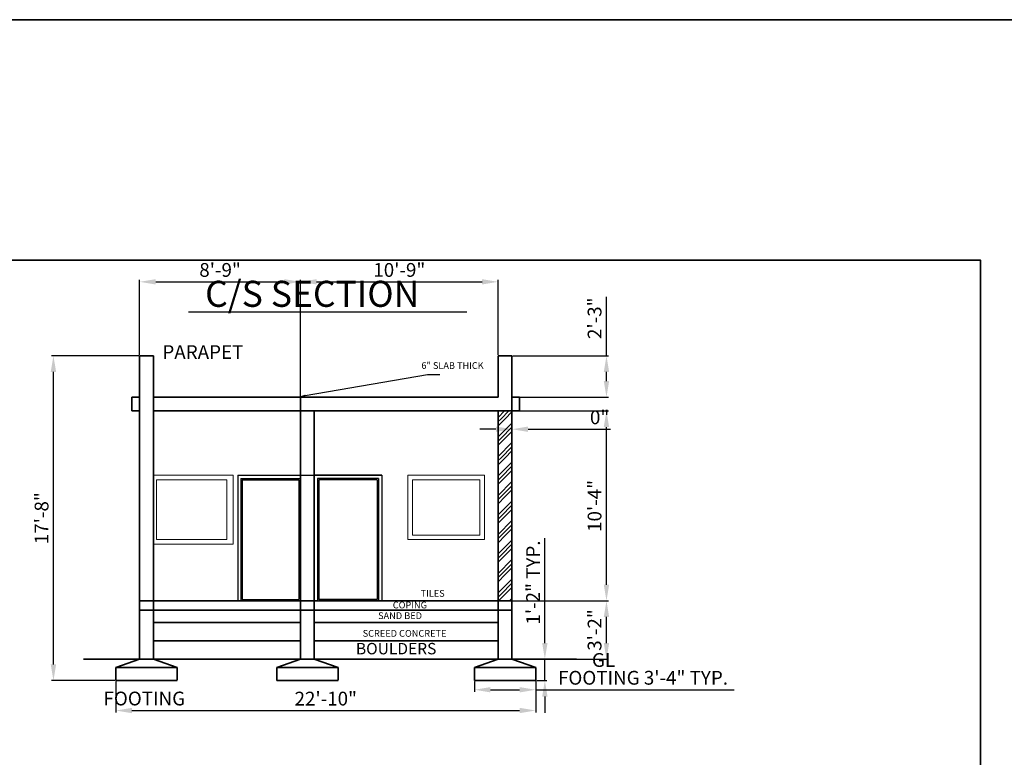
# Model space of a CAD drawing. Units: inches. Extents: x 1956 to 4770, y 1551 to 2596.
# Tile 9 of 10: x 2667 to 3310, y 2115 to 2596. Entities that reach past the tile are written whole.
import ezdxf
from ezdxf import colors
from ezdxf.entities.mleader import LeaderData, LeaderLine
from ezdxf.math import Vec2, Vec3

# ---------------------------------------------------------------- set-up
doc = ezdxf.new("R2010")
doc.units = ezdxf.units.IN
for name, color, linetype, lineweight in [('A-ANNO-DIMS', 2, 'Continuous', 18), ('A-ANNO-TEXT', 7, 'Continuous', 18), ('A-ANNO-TITL', 6, 'Continuous', 25), ('A-ANNO-TTLB', 7, 'Continuous', 35), ('A-DOOR', 3, 'Continuous', 25), ('A-GLAZ', 4, 'Continuous', 18), ('A-SECT', 7, 'Continuous', 35), ('A-SECT-PATT', 8, 'Continuous', 13), ('S-FNDN', 7, 'Continuous', 35)]:
    doc.layers.add(name, color=color, linetype=linetype, lineweight=lineweight)
doc.styles.get("Standard").update_dxf_attribs({"font": 'arial.ttf'})
doc.dimstyles.new('ISO-25', dxfattribs={"dimtxt": 9, "dimasz": 10.5, "dimexe": 1.25, "dimexo": 0.625, "dimgap": 2, "dimtad": 1, "dimdec": 1, "dimlunit": 4, "dimtxsty": 'Standard', "dimcen": 2.5, "dimadec": 0, "dimazin": 0, "dimtfac": 1, "dimtdec": 1, "dimtmove": 0, "dimatfit": 3, "dimfxl": 1, "dimarcsym": 0})

# ---------------------------------------------------------------- blocks, each defined once
blk = doc.blocks.new('*D15')
at = {"layer": 'A-ANNO-DIMS', "color": 0, "lineweight": -2, "transparency": 16777216}
for p, q in [((2988.15, 2340.24), (2988.15, 2327.69)), ((2988.15, 2340.24), (2988.15, 2327.69)), ((2977.65, 2328.94), (2967.15, 2328.94)), ((2998.65, 2328.94), (3052.57, 2328.94))]:
    blk.add_line(p, q, dxfattribs=at)
at = {"layer": 'A-ANNO-DIMS', "color": 0, "transparency": 16777216}
for points in [[(2977.65, 2330.69), (2977.65, 2327.19), (2988.15, 2328.94)], [(2998.65, 2330.69), (2998.65, 2327.19), (2988.15, 2328.94)]]:
    blk.add_solid(points, dxfattribs=at)
at = {"layer": 'Defpoints', "color": 0, "transparency": 16777216}
for p in [(2988.15, 2340.86), (2988.15, 2340.86), (2988.15, 2328.94)]:
    blk.add_point(p, dxfattribs=at)
at = {"layer": 'A-ANNO-DIMS', "color": 0, "transparency": 16777216, "insert": (3045.4, 2335.53), "char_height": 9, "attachment_point": 5}
blk.add_mtext('0"', dxfattribs=at)
blk = doc.blocks.new('FOOTING-40IN-SECTION')
for p, q in [((15.5, 14), (0, 8.58)), ((15.5, 14), (24.5, 14)), ((15.5, 14), (24.5, 14)), ((24.5, 14), (40, 8.58)), ((0, 8.58), (0, 7.18)), ((0, 8.58), (40, 8.58)), ((0, 7.18), (0, 0)), ((40, 8.58), (40, 7.18)), ((40, 7.18), (40, 0.18)), ((0, 0), (40, 0)), ((0, 0), (7.37, 0))]:
    blk.add_line(p, q)
blk = doc.blocks.new('*D37')
at = {"layer": 'A-ANNO-DIMS', "color": 0, "lineweight": -2, "transparency": 16777216}
for p, q in [((2963.65, 2164.24), (2963.65, 2157.61)), ((3003.65, 2164.24), (3003.65, 2157.61)), ((2974.15, 2158.86), (2993.15, 2158.86)), ((3003.65, 2158.86), (3133.27, 2158.86))]:
    blk.add_line(p, q, dxfattribs=at)
at = {"layer": 'A-ANNO-DIMS', "color": 0, "transparency": 16777216}
for points in [[(2974.15, 2160.61), (2974.15, 2157.11), (2963.65, 2158.86)], [(2993.15, 2160.61), (2993.15, 2157.11), (3003.65, 2158.86)]]:
    blk.add_solid(points, dxfattribs=at)
at = {"layer": 'Defpoints', "color": 0, "transparency": 16777216}
for p in [(2963.65, 2164.86), (3003.65, 2164.86), (3003.65, 2158.86)]:
    blk.add_point(p, dxfattribs=at)
at = {"layer": 'A-ANNO-DIMS', "color": 0, "transparency": 16777216, "insert": (3073.71, 2165.52), "char_height": 9, "attachment_point": 5}
blk.add_mtext('FOOTING 3\'-4" TYP.', dxfattribs=at)
blk = doc.blocks.new('*D38')
at = {"layer": 'A-ANNO-DIMS', "color": 0, "lineweight": -2, "transparency": 16777216}
for p, q in [((3009.65, 2189.36), (3009.65, 2257.88)), ((3004.28, 2178.86), (3010.9, 2178.86)), ((3009.65, 2164.86), (3009.65, 2178.86)), ((3004.28, 2164.86), (3010.9, 2164.86)), ((3009.65, 2154.36), (3009.65, 2143.86))]:
    blk.add_line(p, q, dxfattribs=at)
at = {"layer": 'A-ANNO-DIMS', "color": 0, "transparency": 16777216}
for points in [[(3007.9, 2189.36), (3011.4, 2189.36), (3009.65, 2178.86)], [(3007.9, 2154.36), (3011.4, 2154.36), (3009.65, 2164.86)]]:
    blk.add_solid(points, dxfattribs=at)
at = {"layer": 'Defpoints', "color": 0, "transparency": 16777216}
for p in [(3003.65, 2178.86), (3009.65, 2178.86), (3003.65, 2164.86)]:
    blk.add_point(p, dxfattribs=at)
at = {"layer": 'A-ANNO-DIMS', "color": 0, "transparency": 16777216, "insert": (3003.13, 2228.87), "char_height": 9, "attachment_point": 5, "rotation": 90}
blk.add_mtext('1\'-2" TYP.', dxfattribs=at)
blk = doc.blocks.new('*D80')
at = {"layer": 'A-ANNO-DIMS', "color": 0, "lineweight": -2, "transparency": 16777216}
for p, q in [((2729.65, 2164.24), (2729.65, 2144.06)), ((3003.65, 2164.24), (3003.65, 2144.06)), ((2740.15, 2145.31), (2993.15, 2145.31))]:
    blk.add_line(p, q, dxfattribs=at)
at = {"layer": 'A-ANNO-DIMS', "color": 0, "transparency": 16777216}
for points in [[(2740.15, 2147.06), (2740.15, 2143.56), (2729.65, 2145.31)], [(2993.15, 2147.06), (2993.15, 2143.56), (3003.65, 2145.31)]]:
    blk.add_solid(points, dxfattribs=at)
at = {"layer": 'Defpoints', "color": 0, "transparency": 16777216}
for p in [(2729.65, 2164.86), (3003.65, 2164.86), (3003.65, 2145.31)]:
    blk.add_point(p, dxfattribs=at)
at = {"layer": 'A-ANNO-DIMS', "color": 0, "transparency": 16777216, "insert": (2866.65, 2151.91), "char_height": 9, "attachment_point": 5}
blk.add_mtext('22\'-10"', dxfattribs=at)
blk = doc.blocks.new('*D81')
at = {"layer": 'A-ANNO-DIMS', "color": 0, "lineweight": -2, "transparency": 16777216}
for p, q in [((2744.53, 2376.86), (2687.64, 2376.86)), ((2688.89, 2175.36), (2688.89, 2366.36)), ((2729.03, 2164.86), (2687.64, 2164.86))]:
    blk.add_line(p, q, dxfattribs=at)
at = {"layer": 'A-ANNO-DIMS', "color": 0, "transparency": 16777216}
for points in [[(2687.14, 2366.36), (2690.64, 2366.36), (2688.89, 2376.86)], [(2687.14, 2175.36), (2690.64, 2175.36), (2688.89, 2164.86)]]:
    blk.add_solid(points, dxfattribs=at)
at = {"layer": 'Defpoints', "color": 0, "transparency": 16777216}
for p in [(2688.89, 2376.86), (2745.15, 2376.86), (2729.65, 2164.86)]:
    blk.add_point(p, dxfattribs=at)
at = {"layer": 'A-ANNO-DIMS', "color": 0, "transparency": 16777216, "insert": (2682.3, 2270.86), "char_height": 9, "attachment_point": 5, "rotation": 90}
blk.add_mtext('17\'-8"', dxfattribs=at)
blk = doc.blocks.new('*D82')
at = {"layer": 'A-ANNO-DIMS', "color": 0, "lineweight": -2, "transparency": 16777216}
for p, q in [((2988.78, 2340.86), (3051.11, 2340.86)), ((3049.86, 2227.36), (3049.86, 2330.36)), ((2988.78, 2216.86), (3051.11, 2216.86))]:
    blk.add_line(p, q, dxfattribs=at)
at = {"layer": 'A-ANNO-DIMS', "color": 0, "transparency": 16777216}
for points in [[(3048.11, 2330.36), (3051.61, 2330.36), (3049.86, 2340.86)], [(3048.11, 2227.36), (3051.61, 2227.36), (3049.86, 2216.86)]]:
    blk.add_solid(points, dxfattribs=at)
at = {"layer": 'Defpoints', "color": 0, "transparency": 16777216}
for p in [(2988.15, 2340.86), (3049.86, 2340.86), (2988.15, 2216.86)]:
    blk.add_point(p, dxfattribs=at)
at = {"layer": 'A-ANNO-DIMS', "color": 0, "transparency": 16777216, "insert": (3043.27, 2278.86), "char_height": 9, "attachment_point": 5, "rotation": 90}
blk.add_mtext('10\'-4"', dxfattribs=at)
blk = doc.blocks.new('*D83')
at = {"layer": 'A-ANNO-DIMS', "color": 0, "lineweight": -2, "transparency": 16777216}
for p, q in [((3049.86, 2376.86), (3049.86, 2415.44)), ((2988.78, 2376.86), (3051.11, 2376.86)), ((3049.86, 2360.36), (3049.86, 2366.36)), ((2988.78, 2349.86), (3051.11, 2349.86))]:
    blk.add_line(p, q, dxfattribs=at)
at = {"layer": 'A-ANNO-DIMS', "color": 0, "transparency": 16777216}
for points in [[(3048.11, 2366.36), (3051.61, 2366.36), (3049.86, 2376.86)], [(3048.11, 2360.36), (3051.61, 2360.36), (3049.86, 2349.86)]]:
    blk.add_solid(points, dxfattribs=at)
at = {"layer": 'Defpoints', "color": 0, "transparency": 16777216}
for p in [(2988.15, 2376.86), (3049.86, 2376.86), (2988.15, 2349.86)]:
    blk.add_point(p, dxfattribs=at)
at = {"layer": 'A-ANNO-DIMS', "color": 0, "transparency": 16777216, "insert": (3043.26, 2401.4), "char_height": 9, "attachment_point": 5, "rotation": 90}
blk.add_mtext('2\'-3"', dxfattribs=at)
blk = doc.blocks.new('*D84')
at = {"layer": 'A-ANNO-DIMS', "color": 0, "lineweight": -2, "transparency": 16777216}
for p, q in [((2988.78, 2216.86), (3051.11, 2216.86)), ((3049.86, 2189.36), (3049.86, 2206.36)), ((2988.78, 2178.86), (3051.11, 2178.86))]:
    blk.add_line(p, q, dxfattribs=at)
at = {"layer": 'A-ANNO-DIMS', "color": 0, "transparency": 16777216}
for points in [[(3048.11, 2206.36), (3051.61, 2206.36), (3049.86, 2216.86)], [(3048.11, 2189.36), (3051.61, 2189.36), (3049.86, 2178.86)]]:
    blk.add_solid(points, dxfattribs=at)
at = {"layer": 'Defpoints', "color": 0, "transparency": 16777216}
for p in [(2988.15, 2216.86), (3049.86, 2216.86), (2988.15, 2178.86)]:
    blk.add_point(p, dxfattribs=at)
at = {"layer": 'A-ANNO-DIMS', "color": 0, "transparency": 16777216, "insert": (3043.26, 2197.86), "char_height": 9, "attachment_point": 5, "rotation": 90}
blk.add_mtext('3\'-2"', dxfattribs=at)
blk = doc.blocks.new('*D85')
at = {"layer": 'A-ANNO-DIMS', "color": 0, "lineweight": -2, "transparency": 16777216}
for p, q in [((2745.15, 2377.49), (2745.15, 2426.41)), ((2755.65, 2425.16), (2839.65, 2425.16)), ((2850.15, 2350.49), (2850.15, 2426.41))]:
    blk.add_line(p, q, dxfattribs=at)
at = {"layer": 'A-ANNO-DIMS', "color": 0, "transparency": 16777216}
for points in [[(2755.65, 2426.91), (2755.65, 2423.41), (2745.15, 2425.16)], [(2839.65, 2426.91), (2839.65, 2423.41), (2850.15, 2425.16)]]:
    blk.add_solid(points, dxfattribs=at)
at = {"layer": 'Defpoints', "color": 0, "transparency": 16777216}
for p in [(2850.15, 2425.16), (2745.15, 2376.86), (2850.15, 2349.86)]:
    blk.add_point(p, dxfattribs=at)
at = {"layer": 'A-ANNO-DIMS', "color": 0, "transparency": 16777216, "insert": (2797.65, 2431.76), "char_height": 9, "attachment_point": 5}
blk.add_mtext('8\'-9"', dxfattribs=at)
blk = doc.blocks.new('*D86')
at = {"layer": 'A-ANNO-DIMS', "color": 0, "lineweight": -2, "transparency": 16777216}
for p, q in [((2850.15, 2350.49), (2850.15, 2426.41)), ((2860.65, 2425.16), (2968.65, 2425.16)), ((2979.15, 2377.49), (2979.15, 2426.41))]:
    blk.add_line(p, q, dxfattribs=at)
at = {"layer": 'A-ANNO-DIMS', "color": 0, "transparency": 16777216}
for points in [[(2860.65, 2426.91), (2860.65, 2423.41), (2850.15, 2425.16)], [(2968.65, 2426.91), (2968.65, 2423.41), (2979.15, 2425.16)]]:
    blk.add_solid(points, dxfattribs=at)
at = {"layer": 'Defpoints', "color": 0, "transparency": 16777216}
for p in [(2979.15, 2425.16), (2979.15, 2376.86), (2850.15, 2349.86)]:
    blk.add_point(p, dxfattribs=at)
at = {"layer": 'A-ANNO-DIMS', "color": 0, "transparency": 16777216, "insert": (2914.65, 2431.76), "char_height": 9, "attachment_point": 5}
blk.add_mtext('10\'-9"', dxfattribs=at)

msp = doc.modelspace()

# ---------------------------------------------------------------- hatches: boundary and pattern name
at = {"layer": 'A-SECT-PATT'}
h = msp.add_hatch(dxfattribs=at)
h.set_pattern_fill('GOST_GROUND', color=256, scale=0.9)
h.set_pattern_definition([(45, (0, 795.738), (12.727922, 0), [18]), (45, (2.7, 795.738), (12.727922, 0), [18]), (45, (5.4, 795.738), (12.727922, 0), [18])])
h.paths.add_polyline_path([(2988.15, 2340.86), (2979.15, 2340.86), (2979.15, 2216.86), (2988.15, 2216.86)])

# ---------------------------------------------------------------- linework, layer by layer
at = {"layer": 'A-ANNO-TITL'}
msp.add_line((2776.95, 2405.61), (2958.68, 2405.61), dxfattribs=at)
at = {"layer": 'A-ANNO-TTLB'}
for points in [[(1955.79, 2596.29), (4769.89, 2596.29), (4769.89, 1551.4), (1955.79, 1551.4)], [(2042.64, 2439.33), (3293.93, 2439.33), (3293.93, 1676.04), (2042.64, 1676.04)]]:
    msp.add_lwpolyline(points, close=True, dxfattribs=at)
at = {"layer": 'A-DOOR'}
for p, q in [((2809.15, 2298.86), (2850.15, 2298.86)), ((2809.15, 2298.86), (2809.15, 2216.86)), ((2809.15, 2298.86), (2809.15, 2216.86)), ((2809.15, 2298.86), (2903.15, 2298.86)), ((2811.15, 2296.86), (2850.15, 2296.86)), ((2811.15, 2296.86), (2811.15, 2216.86)), ((2812.15, 2295.86), (2849.15, 2295.86)), ((2812.15, 2295.86), (2812.15, 2217.86)), ((2849.15, 2295.86), (2849.15, 2217.86)), ((2903.15, 2298.86), (2859.15, 2298.86)), ((2901.15, 2296.86), (2861.15, 2296.86)), ((2861.15, 2296.86), (2861.15, 2216.86)), ((2862.15, 2295.86), (2862.15, 2217.86)), ((2900.15, 2295.86), (2862.15, 2295.86)), ((2900.15, 2295.86), (2900.15, 2217.86)), ((2901.15, 2296.86), (2901.15, 2216.86)), ((2903.15, 2298.86), (2903.15, 2216.86)), ((2812.15, 2217.86), (2849.15, 2217.86)), ((2900.15, 2217.86), (2862.15, 2217.86)), ((2861.15, 2216.86), (2901.15, 2216.86))]:
    msp.add_line(p, q, dxfattribs=at)
at = {"layer": 'A-GLAZ'}
for p, q in [((2754.15, 2298.86), (2806.15, 2298.86)), ((2756.15, 2295.86), (2802.15, 2295.86)), ((2756.15, 2295.86), (2756.15, 2256.86)), ((2758.15, 2298.86), (2806.15, 2298.86)), ((2802.15, 2295.86), (2802.15, 2256.86)), ((2806.15, 2298.86), (2806.15, 2253.86)), ((2920.15, 2298.86), (2920.15, 2256.86)), ((2920.15, 2298.86), (2920.15, 2256.86)), ((2920.15, 2298.86), (2970.15, 2298.86)), ((2923.15, 2295.86), (2967.15, 2295.86)), ((2923.15, 2295.86), (2923.15, 2259.86)), ((2967.15, 2295.86), (2967.15, 2259.86)), ((2970.15, 2298.86), (2970.15, 2256.86)), ((2756.15, 2256.86), (2802.15, 2256.86)), ((2920.15, 2256.86), (2970.15, 2256.86)), ((2923.15, 2259.86), (2967.15, 2259.86)), ((2754.15, 2253.86), (2806.15, 2253.86))]:
    msp.add_line(p, q, dxfattribs=at)
at = {"layer": 'A-SECT'}
for p, q in [((2745.15, 2376.86), (2745.15, 2340.86)), ((2745.15, 2376.86), (2754.15, 2376.86)), ((2754.15, 2376.86), (2754.15, 2349.86)), ((2979.15, 2376.86), (2979.15, 2349.86)), ((2979.15, 2376.86), (2988.15, 2376.86)), ((2988.15, 2376.86), (2988.15, 2340.86)), ((2740.15, 2349.86), (2745.15, 2349.86)), ((2740.15, 2349.86), (2740.15, 2340.86)), ((2754.15, 2349.86), (2754.15, 2178.86)), ((2754.15, 2349.86), (2979.15, 2349.86)), ((2850.15, 2349.86), (2850.15, 2216.86)), ((2988.15, 2349.86), (2993.15, 2349.86)), ((2993.15, 2349.86), (2993.15, 2340.86)), ((2740.15, 2340.86), (2745.15, 2340.86)), ((2745.15, 2340.86), (2745.15, 2178.86)), ((2754.15, 2340.86), (2988.15, 2340.86)), ((2859.15, 2340.86), (2859.15, 2216.86)), ((2979.15, 2340.86), (2979.15, 2178.86)), ((2988.15, 2340.86), (2993.15, 2340.86)), ((2988.15, 2340.86), (2988.15, 2178.86)), ((2850.15, 2298.86), (2850.15, 2178.86)), ((2859.15, 2298.86), (2859.15, 2178.86)), ((2745.15, 2216.86), (2861.15, 2216.86)), ((2745.15, 2210.86), (2988.15, 2210.86)), ((2745.15, 2210.86), (2812.15, 2210.86)), ((2988.15, 2216.86), (2862.15, 2216.86)), ((2754.15, 2202.86), (2850.15, 2202.86)), ((2859.15, 2202.86), (2979.15, 2202.86)), ((2754.15, 2190.86), (2850.15, 2190.86)), ((2859.15, 2190.86), (2979.15, 2190.86)), ((2708.44, 2178.86), (3030.31, 2178.86))]:
    msp.add_line(p, q, dxfattribs=at)

# ---------------------------------------------------------------- block references
at = {"layer": 'S-FNDN'}
for p in [(2729.65, 2164.86), (2834.65, 2164.86), (2963.65, 2164.86)]:
    msp.add_blockref('FOOTING-40IN-SECTION', p, dxfattribs=at)

# ---------------------------------------------------------------- texts
at = {"layer": 'A-ANNO-TEXT'}
for s, height, p in [(' PARAPET ', 9, (2757.24, 2374.81)), ('TILES ', 4.399, (2928.53, 2219.56)), (' COPING ', 4.399, (2909.04, 2211.97)), (' SAND BED ', 4.399, (2899.46, 2205.02)), (' SCREED CONCRETE ', 4.3995, (2889.39, 2193.46)), (' BOULDERS ', 7.442, (2884.05, 2181.98)), (' GL ', 9, (3037.64, 2173.79)), (' FOOTING ', 9, (2718.81, 2148.64))]:
    msp.add_text(s, height=height, dxfattribs=at).set_placement(p)
at = {"layer": 'A-ANNO-TEXT', "insert": (2929.1, 2372.71), "char_height": 4.384, "attachment_point": 1}
msp.add_mtext_dynamic_manual_height_columns('6" SLAB THICK', width=44.3756, gutter_width=21.92, heights=[0], dxfattribs=at)
at = {"layer": 'A-ANNO-TITL'}
msp.add_text(' C/S SECTION ', height=17, dxfattribs=at).set_placement((2782.68, 2408.83))

# ---------------------------------------------------------------- dimensions: what is measured, and where the dimension line sits
at = {"layer": 'A-ANNO-DIMS'}
for base, p1, p2, picture, middle in [((2850.15, 2425.16), (2745.15, 2376.86), (2850.15, 2349.86), '*D85', (2797.65, 2431.76)), ((2979.15, 2425.16), (2850.15, 2349.86), (2979.15, 2376.86), '*D86', (2914.65, 2431.76)), ((3003.65, 2145.31), (2729.65, 2164.86), (3003.65, 2164.86), '*D80', (2866.65, 2151.91))]:
    dim = msp.add_linear_dim(base=base, p1=p1, p2=p2, dimstyle='ISO-25', override={"dimdec": 1, "dimlfac": 1, "dimrnd": 0, "dimzin": 1, "dimdsep": 46, "dimlunit": 4, "dimfrac": 2}, dxfattribs=at)
    dim.commit()
    dim.dimension.update_dxf_attribs({"geometry": picture, "text_midpoint": middle})
for base, p1, p2, picture, middle in [((3049.86, 2376.86), (2988.15, 2349.86), (2988.15, 2376.86), '*D83', (3043.26, 2401.4)), ((2688.89, 2376.86), (2729.65, 2164.86), (2745.15, 2376.86), '*D81', (2682.3, 2270.86)), ((3049.86, 2340.86), (2988.15, 2216.86), (2988.15, 2340.86), '*D82', (3043.27, 2278.86)), ((3049.86, 2216.86), (2988.15, 2178.86), (2988.15, 2216.86), '*D84', (3043.26, 2197.86))]:
    dim = msp.add_linear_dim(base=base, p1=p1, p2=p2, angle=90, dimstyle='ISO-25', override={"dimdec": 1, "dimlfac": 1, "dimrnd": 0, "dimzin": 1, "dimdsep": 46, "dimlunit": 4, "dimfrac": 2}, dxfattribs=at)
    dim.commit()
    dim.dimension.update_dxf_attribs({"geometry": picture, "text_midpoint": middle})
dim = msp.add_linear_dim(base=(2988.1542495, 2328.9357667), p1=(2988.1542495, 2340.86408281), p2=(2988.1542495, 2340.86408281), dimstyle='ISO-25', override={"dimclrd": 0, "dimclre": 0, "dimclrt": 0}, dxfattribs=at)
dim.commit()
dim.dimension.update_dxf_attribs({"geometry": '*D15', "text_midpoint": (3045.39538183, 2328.9357667), "dimtype": 160})
dim = msp.add_linear_dim(base=(3009.65, 2178.86), p1=(3003.65, 2164.86), p2=(3003.65, 2178.86), angle=90, text='<> TYP.', dimstyle='ISO-25', override={"dimdec": 1, "dimlfac": 1, "dimrnd": 0, "dimzin": 1, "dimdsep": 46, "dimlunit": 4, "dimfrac": 2}, dxfattribs=at)
dim.commit()
dim.dimension.update_dxf_attribs({"geometry": '*D38', "text_midpoint": (3003.13, 2228.87)})
dim = msp.add_linear_dim(base=(3003.65, 2158.86), p1=(2963.65, 2164.86), p2=(3003.65, 2164.86), text='FOOTING <> TYP.', dimstyle='ISO-25', override={"dimdec": 1, "dimlfac": 1, "dimrnd": 0, "dimzin": 1, "dimdsep": 46, "dimlunit": 4, "dimfrac": 2}, dxfattribs=at)
dim.commit()
dim.dimension.update_dxf_attribs({"geometry": '*D37', "text_midpoint": (3073.71, 2165.52)})

# ---------------------------------------------------------------- leaders
at = {"layer": 'A-ANNO-TEXT'}
ml = msp.add_multileader_mtext('Standard', dxfattribs=at)
ml.set_content('', color=256)
ml.set_leader_properties()
ml.build(insert=Vec2(0, 0))
ctx = ml.context
ctx.base_point, ctx.plane_origin = Vec3(2941, 2364.6), Vec3(2849.36, 2350.2)
notes = []
notes.append((ctx, [(0, (1, 1, 0), (2933, 2364.6), (1, 0), 8, [(0, [(2849.36, 2350.2)], 0, [])])]))
ctx.mtext.insert, ctx.mtext.flow_direction = Vec3(2943, 2366.6), 5
for ctx, leaders in notes:
    for number, flags, end, landing, length, lines in leaders:
        leader = LeaderData()
        leader.index, (leader.has_last_leader_line, leader.has_dogleg_vector, leader.attachment_direction) = number, flags
        leader.last_leader_point, leader.dogleg_vector, leader.dogleg_length = Vec3(end), Vec3(landing), length
        for number, points, colour, breaks in lines:
            line = LeaderLine()
            line.index, line.vertices, line.color, line.breaks = number, Vec3.list(points), colors.encode_raw_color(colour), breaks
            leader.lines.append(line)
        ctx.leaders.append(leader)

doc.saveas('drawing.dxf')
